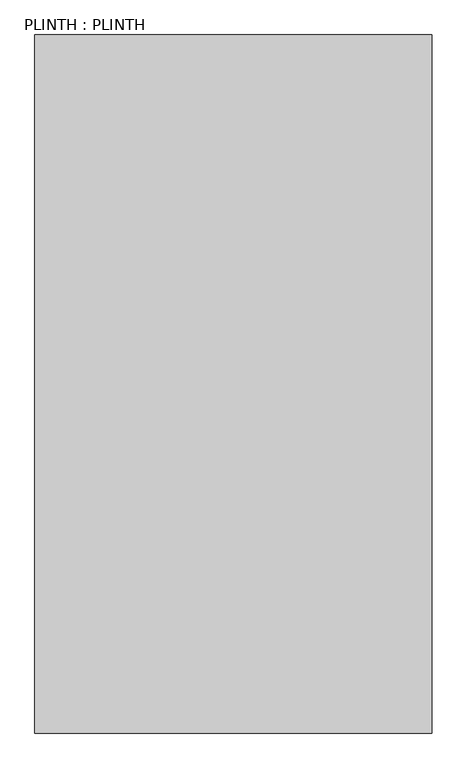
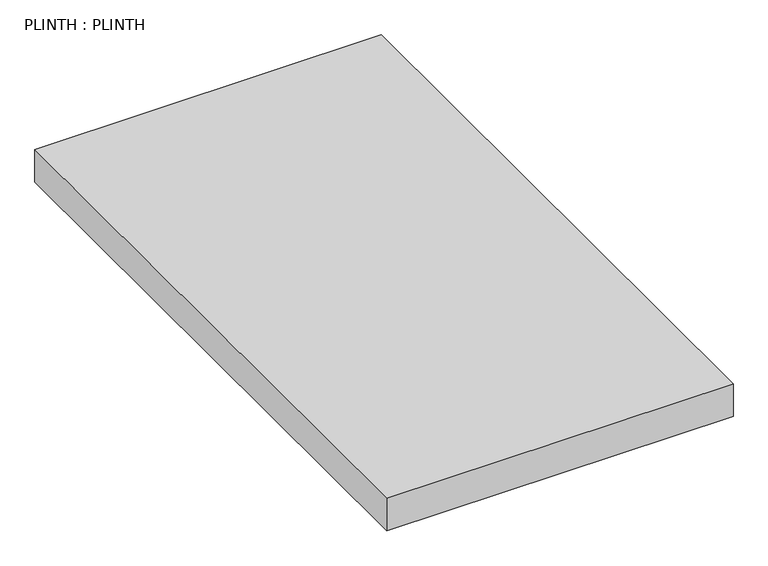
"""IFC4 building model written with IfcOpenShell, lengths in millimetres: proxy geometry, PLINTH : PLINTH."""

from ifc_helpers import new_model, si_unit, origin, origin_with_axes, place, context, project, spatial, polyline, outline, extrude, source, transform, mapped, element, save


def plinth_plinth_0a88a6c8(model_context):
    return source(origin(), model_context, "Body", "SweptSolid", [
        extrude(outline(polyline([(-23811.2963079, 6326.0742053), (-17639.0963079, 6326.0742053), (-17639.0963079, -4519.7257947), (-23811.2963079, -4519.7257947), (-23811.2963079, 6326.0742053)])), origin_with_axes(), (0.0, 0.0, 1.0), 609.6),
    ])


if __name__ == "__main__":
    model = new_model("IFC4")
    model_context = context("Model", 3, world=origin())
    ifc_project = project(units=[si_unit("LENGTHUNIT", "METRE", prefix="MILLI")], contexts=[model_context])
    site = spatial("IfcSite", under=ifc_project)
    building = spatial("IfcBuilding", under=site)
    placement = place(None, origin())
    plinth_plinth_shape = plinth_plinth_0a88a6c8(model_context)
    element("IfcBuildingElementProxy", 1, Name="PLINTH : PLINTH", ObjectType="PLINTH : PLINTH", at=placement, inside=building, context=model_context, shape_type="MappedRepresentation", body=[
        mapped(plinth_plinth_shape, transform((0.0, 0.0, 0.0), x_axis=(1.0, 0.0, 0.0), y_axis=(0.0, 1.0, 0.0), z_axis=(0.0, 0.0, 1.0))),
    ])
    save(model, "model.ifc")
